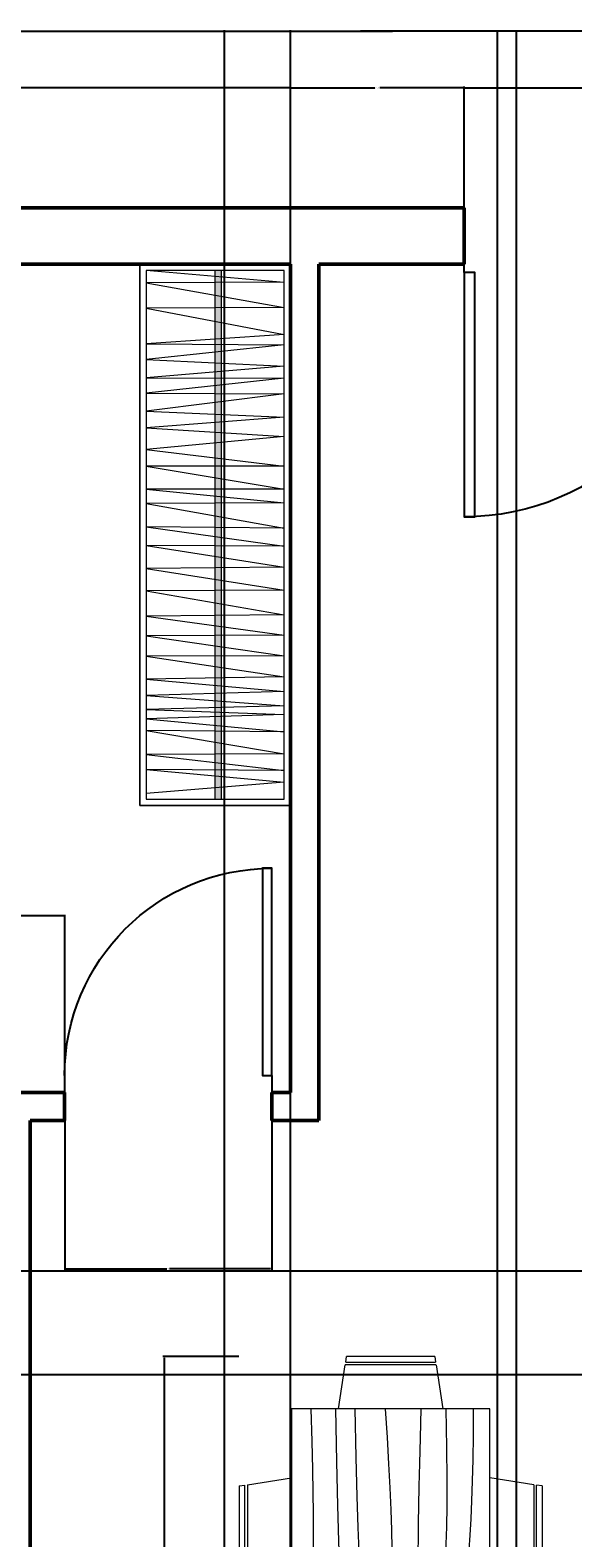
# Model space of a CAD drawing. Units: inches. Extents: x 1974 to 2406, y 1583 to 2170.
# Tile 5 of 6: x 2138 to 2224, y 1930 to 2170. Entities that reach past the tile are written whole.
import ezdxf

# ---------------------------------------------------------------- set-up
doc = ezdxf.new("R2010")
doc.units = ezdxf.units.IN
for name, color, linetype, lineweight in [('A-ANNO-DIMS', 2, 'Continuous', 18), ('A-FURN', 3, 'Continuous', 18), ('door', 60, 'Continuous', 25), ('wall', 240, 'Continuous', 50)]:
    doc.layers.add(name, color=color, linetype=linetype, lineweight=lineweight)
doc.layers.add('A-FLOR-CASE', color=40, linetype='Continuous', lineweight=18, true_color=0xf8d731)
doc.layers.add('A-FLOR-CASE-PATT', color=40, linetype='Continuous', lineweight=13, true_color=0xf8d731)
doc.styles.get("Standard").update_dxf_attribs({"font": 'arial.ttf'})
doc.dimstyles.get("Standard").update_dxf_attribs({"dimtxt": 0.18, "dimasz": 0.18, "dimexe": 0.18, "dimexo": 0.0625, "dimgap": 0.09, "dimtad": 0, "dimtih": 1, "dimtoh": 1, "dimdec": 4, "dimzin": 0, "dimdsep": 46, "dimtxsty": 'Standard', "dimcen": 0.09, "dimadec": 0, "dimazin": 0, "dimtfac": 1, "dimtdec": 4, "dimtofl": 0, "dimtmove": 0, "dimatfit": 3, "dimfxl": 1, "dimtolj": 1, "dimtzin": 0, "dimarcsym": 0})

# ---------------------------------------------------------------- blocks, each defined once
blk = doc.blocks.new('*U2')
for p, q in [((0, 0), (0, -6)), ((40, 0), (40, -6))]:
    blk.add_line(p, q)
blk.add_lwpolyline([(0, 0), (0, 40), (1.75, 40), (1.75, 0)], close=True)
blk.add_arc((0, 0), 40, 0, 90)
blk = doc.blocks.new('Dining Set - 36 x 72 in.')
for p, q in [((-22, 27.5), (-22.1562, 26.50042)), ((-22, 27.5), (-6, 27.5)), ((-5.8437, 26.49966), (-6, 27.5)), ((6, 27.5), (5.8438, 26.50042)), ((6, 27.5), (22, 27.5)), ((22.1563, 26.49966), (22, 27.5)), ((-22.2343, 26.00059), (-23.4847, 17.99762)), ((-22.2304, 26), (-5.7608, 26)), ((-5.8416, 26.5), (-22.1534, 26.5)), ((-4.5152, 17.99762), (-5.7655, 25.99926)), ((5.7657, 26.00059), (4.5153, 17.99762)), ((5.7696, 26), (22.2392, 26)), ((22.1584, 26.5), (5.8466, 26.5)), ((23.4848, 17.99762), (22.2345, 25.99926)), ((36, 18), (-36, 18)), ((-36, 18), (-36, -18)), ((36, -18), (36, 18)), ((-44.0006, 8.23428), (-35.9976, 9.48474)), ((-44, 8.23041), (-44, -8.23915)), ((44.0006, 8.23428), (35.9976, 9.48474)), ((44, 8.23041), (44, -8.23915)), ((-45.5, 8), (-44.5004, 8.15617)), ((-45.5, 8), (-45.5, -8)), ((-44.5, -8.15843), (-44.5, 8.15338)), ((44.5, -8.15843), (44.5, 8.15338)), ((45.5, 8), (44.5005, 8.15617)), ((45.5, 8), (45.5, -8)), ((-44.4997, -8.15631), (-45.5, -8)), ((44.4997, -8.15631), (45.5, -8)), ((-35.9976, -9.48476), (-43.9993, -8.2345)), ((35.9976, -9.48476), (43.9993, -8.2345)), ((-36, -18), (36, -18)), ((-22.2343, -26.0006), (-23.4847, -17.99762)), ((-4.5152, -17.99762), (-5.7655, -25.99928)), ((5.7657, -26.0006), (4.5153, -17.99762)), ((23.4848, -17.99762), (22.2345, -25.99928)), ((-22.2304, -26), (-5.7608, -26)), ((-22, -27.5), (-22.1562, -26.50044)), ((-5.8416, -26.5), (-22.1534, -26.5)), ((-5.8437, -26.49967), (-6, -27.5)), ((5.7696, -26), (22.2392, -26)), ((6, -27.5), (5.8438, -26.50044)), ((22.1584, -26.5), (5.8466, -26.5)), ((22.1563, -26.49967), (22, -27.5)), ((-22, -27.5), (-6, -27.5)), ((6, -27.5), (22, -27.5))]:
    blk.add_line(p, q)
for points in [[(-36, 15), (-31.1772, 14.97754), (-26.8079, 14.91406), (-22.8538, 14.81543), (-19.276, 14.6875), (-16.0362, 14.53613), (-13.0957, 14.36718), (-10.4159, 14.18652), (-7.9583, 14), (-5.6904, 13.81315), (-3.6035, 13.63021), (-1.6954, 13.45508), (0.0365, 13.29166), (1.5945, 13.14388), (2.9811, 13.01562), (4.1988, 12.9108), (5.25, 12.83333), (6.1393, 12.78613), (6.8802, 12.76823), (7.4883, 12.77767), (7.9792, 12.8125), (8.3685, 12.87077), (8.6719, 12.95052), (8.9049, 13.0498), (9.0833, 13.16666), (9.2205, 13.29899), (9.3216, 13.44401), (9.3895, 13.59879), (9.4271, 13.76041), (9.4373, 13.92594), (9.4232, 14.09245), (9.3875, 14.257), (9.3333, 14.41666), (9.2638, 14.56917), (9.1836, 14.71484), (9.0975, 14.85465), (9.0104, 14.98958), (8.9272, 15.1206), (8.8529, 15.2487), (8.7922, 15.37483), (8.75, 15.5), (8.7305, 15.62467), (8.7344, 15.74739), (8.7617, 15.86621), (8.8125, 15.97916), (8.8867, 16.08431), (8.9844, 16.17968), (9.1055, 16.26334), (9.25, 16.33333), (9.4189, 16.38802), (9.6172, 16.42708), (9.8506, 16.45052), (10.125, 16.45833), (10.4463, 16.45052), (10.8203, 16.42708), (11.2529, 16.38802), (11.75, 16.33333), (12.3184, 16.26318), (12.9694, 16.17838), (13.7151, 16.07991), (14.5677, 15.96875), (15.5395, 15.84586), (16.6426, 15.71224), (17.8893, 15.56884), (19.2917, 15.41666), (20.859, 15.25667), (22.5879, 15.08984), (24.4721, 14.91715), (26.5052, 14.73958), (28.6809, 14.5581), (30.9929, 14.3737), (33.4347, 14.18733), (36, 14)], [(-36, 10), (-28.9766, 10.14274), (-23.1725, 10.20442), (-18.4241, 10.19775), (-14.5677, 10.13541), (-11.4399, 10.03011), (-8.877, 9.89453), (-6.7154, 9.74137), (-4.7917, 9.58333), (-2.9698, 9.43082), (-1.2246, 9.28515), (0.4415, 9.14534), (2.026, 9.01041), (3.5266, 8.87939), (4.9408, 8.7513), (6.266, 8.62516), (7.5, 8.5), (8.6411, 8.37549), (9.6914, 8.2539), (10.6538, 8.13818), (11.5312, 8.03125), (12.3267, 7.93603), (13.043, 7.85547), (13.6831, 7.79248), (14.25, 7.75), (14.7471, 7.7303), (15.1797, 7.73307), (15.5537, 7.75732), (15.875, 7.80208), (16.1494, 7.86637), (16.3828, 7.94922), (16.5811, 8.04964), (16.75, 8.16666), (16.8944, 8.29915), (17.0143, 8.44531), (17.1089, 8.60319), (17.1771, 8.77083), (17.218, 8.94629), (17.2305, 9.1276), (17.2137, 9.31282), (17.1667, 9.5), (17.0895, 9.6875), (16.987, 9.875), (16.8649, 10.0625), (16.7292, 10.25), (16.5856, 10.4375), (16.4401, 10.625), (16.2985, 10.8125), (16.1667, 11), (16.05, 11.18733), (15.9518, 11.3737), (15.8752, 11.5581), (15.8229, 11.73958), (15.798, 11.91715), (15.8034, 12.08984), (15.842, 12.25667), (15.9167, 12.41666), (16.0295, 12.56836), (16.1784, 12.70833), (16.3605, 12.83268), (16.5729, 12.9375), (16.8127, 13.01888), (17.0768, 13.07291), (17.3625, 13.0957), (17.6667, 13.08333), (17.9894, 13.03312), (18.3418, 12.94726), (18.7382, 12.82918), (19.1927, 12.68229), (19.7195, 12.51001), (20.3327, 12.31575), (21.0465, 12.10294), (21.875, 11.875), (22.8357, 11.63354), (23.959, 11.37304), (25.2786, 11.08618), (26.8282, 10.76562), (28.6414, 10.40405), (30.752, 9.99414), (33.1936, 9.52856), (36, 9)], [(-36, 5.5), (-30.7157, 5.3348), (-26.069, 5.20963), (-21.9946, 5.11767), (-18.4271, 5.05208), (-15.3009, 5.00602), (-12.5508, 4.97265), (-10.1112, 4.94515), (-7.9167, 4.91666), (-5.909, 4.88167), (-4.0586, 4.83984), (-2.3429, 4.79215), (-0.7396, 4.73958), (0.7739, 4.6831), (2.22, 4.6237), (3.6213, 4.56233), (5, 4.5), (6.373, 4.43782), (7.7344, 4.3776), (9.0723, 4.32129), (10.375, 4.27083), (11.6309, 4.22819), (12.8281, 4.19531), (13.9551, 4.17415), (15, 4.16666), (15.954, 4.17448), (16.819, 4.19791), (17.6001, 4.23698), (18.3021, 4.29166), (18.9299, 4.36198), (19.4883, 4.44791), (19.9823, 4.54948), (20.4167, 4.66666), (20.7969, 4.79899), (21.1302, 4.94401), (21.4245, 5.09879), (21.6875, 5.26041), (21.9271, 5.42594), (22.1511, 5.59245), (22.3672, 5.757), (22.5834, 5.91666), (22.8065, 6.06868), (23.0404, 6.21093), (23.2879, 6.34147), (23.5521, 6.45833), (23.8358, 6.55957), (24.142, 6.64323), (24.4735, 6.70735), (24.8334, 6.75), (25.2235, 6.76969), (25.642, 6.76692), (26.0858, 6.74267), (26.5521, 6.69791), (27.0379, 6.63362), (27.5404, 6.55078), (28.0565, 6.45036), (28.5834, 6.33333), (29.1242, 6.19987), (29.7071, 6.04687), (30.3661, 5.87044), (31.1354, 5.66666), (32.0493, 5.43164), (33.142, 5.16146), (34.4475, 4.85221), (36, 4.5)], [(-36, -1), (-30.7915, -0.6591), (-26.0195, -0.38216), (-21.6519, -0.16284), (-17.6563, 0.00521), (-14.0005, 0.12833), (-10.6523, 0.21289), (-7.5796, 0.26522), (-4.75, 0.29166), (-2.134, 0.29793), (0.2878, 0.28711), (2.5317, 0.26163), (4.6146, 0.22396), (6.5529, 0.17651), (8.3633, 0.12174), (10.0623, 0.06209), (11.6667, 0), (13.1899, -0.06201), (14.6341, -0.1211), (15.9982, -0.17432), (17.2813, -0.21875), (18.4823, -0.25147), (19.6003, -0.26953), (20.6343, -0.27002), (21.5834, -0.25), (22.4481, -0.20768), (23.2357, -0.14584), (23.9549, -0.06836), (24.6146, 0.02083), (25.2235, 0.11784), (25.7904, 0.21875), (26.3241, 0.31966), (26.8334, 0.41666), (27.3265, 0.50618), (27.8099, 0.58593), (28.2894, 0.65397), (28.7709, 0.70833), (29.2601, 0.74707), (29.763, 0.76823), (30.2855, 0.76985), (30.8334, 0.75), (31.4088, 0.70784), (31.9994, 0.64713), (32.589, 0.57275), (33.1615, 0.48958), (33.7008, 0.4025), (34.1908, 0.3164), (34.6153, 0.23616), (34.9584, 0.16666), (35.2099, 0.11165), (35.3848, 0.07031), (35.504, 0.04069), (35.5886, 0.02083), (35.6594, 0.00879), (35.7377, 0.0026), (35.8442, 0.00032), (36, 0)], [(-36, -6.5), (-27.1843, -6.31267), (-20.084, -6.1263), (-14.469, -5.9419), (-10.1094, -5.76042), (-6.7752, -5.58285), (-4.2363, -5.41016), (-2.2629, -5.24333), (-0.625, -5.08334), (0.8708, -4.93099), (2.2715, -4.78646), (3.5872, -4.64974), (4.8281, -4.52084), (6.0046, -4.39974), (7.127, -4.28646), (8.2053, -4.18099), (9.25, -4.08334), (10.2705, -3.99382), (11.2734, -3.91407), (12.2647, -3.84603), (13.25, -3.79167), (14.2354, -3.75293), (15.2266, -3.73177), (16.2295, -3.73015), (17.25, -3.75), (18.2912, -3.79248), (19.3451, -3.85547), (20.4009, -3.93604), (21.4479, -4.03125), (22.4754, -4.13819), (23.4727, -4.25391), (24.4289, -4.37549), (25.3334, -4.5), (26.1785, -4.62492), (26.9694, -4.74935), (27.7145, -4.87281), (28.4219, -4.99479), (29.1, -5.11483), (29.7572, -5.23242), (30.4016, -5.34709), (31.0417, -5.45834), (31.6837, -5.56437), (32.3262, -5.65821), (32.9658, -5.73153), (33.599, -5.77604), (34.2224, -5.78345), (34.8327, -5.74545), (35.4264, -5.65373), (36, -5.5)], [(-36, -10), (-26.4022, -9.81299), (-18.4675, -9.62891), (-11.9839, -9.45069), (-6.7396, -9.28125), (-2.5226, -9.12354), (0.8789, -8.98047), (3.6769, -8.85498), (6.0833, -8.75), (8.2767, -8.66765), (10.3021, -8.60677), (12.1712, -8.56543), (13.8958, -8.54167), (15.4876, -8.53353), (16.9583, -8.53907), (18.3197, -8.55632), (19.5834, -8.58334), (20.7616, -8.61841), (21.8685, -8.66081), (22.9188, -8.71004), (23.9271, -8.76563), (24.9081, -8.82707), (25.8763, -8.89388), (26.8465, -8.96558), (27.8334, -9.04167), (28.8474, -9.12118), (29.8828, -9.20117), (30.93, -9.27824), (31.9792, -9.34896), (33.0205, -9.40991), (34.0443, -9.45768), (35.0407, -9.48885), (36, -9.5)], [(-36, -14.5), (-30.0881, -14.33513), (-25.0332, -14.21224), (-20.7312, -14.12647), (-17.0781, -14.07292), (-13.97, -14.04671), (-11.3027, -14.04297), (-8.9724, -14.05681), (-6.875, -14.08334), (-4.9224, -14.11833), (-3.0905, -14.16016), (-1.3709, -14.20785), (0.2448, -14.26042), (1.7647, -14.3169), (3.1973, -14.3763), (4.5507, -14.43767), (5.8333, -14.5), (7.0554, -14.5621), (8.235, -14.62175), (9.3922, -14.67652), (10.5469, -14.72396), (11.7192, -14.76164), (12.929, -14.78711), (14.1965, -14.79794), (15.5417, -14.79167), (16.9933, -14.76424), (18.6152, -14.70508), (20.4804, -14.60197), (22.6615, -14.44271), (25.2312, -14.21509), (28.2624, -13.9069), (31.8277, -13.50594), (36, -13)]]:
    blk.add_lwpolyline(points)
blk = doc.blocks.new('CLOSET-HANGER-RUN')
for p, q in [((0, 0), (0, 22)), ((0.94, 0), (2.86, 22)), ((2.86, 22), (2.99, 0)), ((2.99, 0), (6.93, 22)), ((6.93, 22), (6.99, 0)), ((6.99, 0), (11.19, 22)), ((11.19, 22), (12.71, 0)), ((12.71, 0), (12.83, 22)), ((12.83, 22), (15.2, 0)), ((15.2, 0), (16.24, 22)), ((16.24, 22), (18.1, 0)), ((18.1, 0), (18.16, 22)), ((18.16, 22), (20.55, 0)), ((20.55, 0), (20.68, 22)), ((20.68, 22), (23.44, 0)), ((23.44, 0), (24.36, 22)), ((24.36, 22), (26.08, 0)), ((26.08, 0), (27.44, 22)), ((27.44, 22), (29.52, 0)), ((29.52, 0), (32.2, 22)), ((32.2, 22), (32.2, 0)), ((32.2, 0), (35.87, 22)), ((35.87, 22), (35.87, 0)), ((35.87, 0), (38.02, 22)), ((38.02, 22), (38.12, 0)), ((38.12, 0), (42.07, 22)), ((42.07, 22), (41.87, 0)), ((41.87, 0), (44.93, 22)), ((44.93, 22), (44.83, 0)), ((44.83, 0), (48.29, 22)), ((48.29, 22), (48.48, 0)), ((48.48, 0), (51.94, 22)), ((51.94, 22), (52.04, 0)), ((52.04, 0), (55.89, 22)), ((55.89, 22), (56.08, 0)), ((56.08, 0), (59.14, 22)), ((59.14, 22), (59.24, 0)), ((59.24, 0), (62.4, 22)), ((62.4, 22), (62.5, 0)), ((62.5, 0), (65.76, 22)), ((65.76, 22), (66.15, 0)), ((66.15, 0), (68.13, 22)), ((68.13, 22), (68.72, 0)), ((68.72, 0), (70.4, 22)), ((70.4, 22), (70.99, 0)), ((70.99, 0), (71.78, 22)), ((71.78, 22), (72.44, 0))]:
    blk.add_line(p, q)
blk = doc.blocks.new('*D42')
at = {"layer": 'A-ANNO-DIMS', "color": 0, "lineweight": -2, "transparency": 16777216}
for p, q in [((2170.92, 1958.88), (2158.82, 1958.88)), ((2159, 1958.7), (2159, 1919.13)), ((2159, 1879.18), (2159, 1918.76)), ((2170.92, 1879), (2158.82, 1879))]:
    blk.add_line(p, q, dxfattribs=at)
at = {"layer": 'A-ANNO-DIMS', "color": 0, "transparency": 16777216}
for points in [[(2158.97, 1958.7), (2159.03, 1958.7), (2159, 1958.88)], [(2158.97, 1879.18), (2159.03, 1879.18), (2159, 1879)]]:
    blk.add_solid(points, dxfattribs=at)
at = {"layer": 'Defpoints', "color": 0, "transparency": 16777216}
for p in [(2170.98, 1958.88), (2159, 1879), (2170.98, 1879)]:
    blk.add_point(p, dxfattribs=at)
at = {"layer": 'A-ANNO-DIMS', "color": 0, "transparency": 16777216, "insert": (2159, 1918.94), "char_height": 0.18, "attachment_point": 5}
blk.add_mtext('\\A1;DINING SET 80', dxfattribs=at)
blk = doc.blocks.new('*D48')
at = {"layer": 'A-ANNO-DIMS', "color": 0, "lineweight": -2, "transparency": 16777216}
for p, q in [((2002.16, 2142.05), (2002.16, 2170.29)), ((2002.34, 2170.11), (2189.51, 2170.11)), ((2377.48, 2170.11), (2190.3, 2170.11)), ((2377.66, 2142.05), (2377.66, 2170.29))]:
    blk.add_line(p, q, dxfattribs=at)
at = {"layer": 'A-ANNO-DIMS', "color": 0, "transparency": 16777216}
for points in [[(2002.34, 2170.14), (2002.34, 2170.08), (2002.16, 2170.11)], [(2377.48, 2170.14), (2377.48, 2170.08), (2377.66, 2170.11)]]:
    blk.add_solid(points, dxfattribs=at)
at = {"layer": 'Defpoints', "color": 0, "transparency": 16777216}
for p in [(2377.66, 2170.11), (2002.16, 2141.99), (2377.66, 2141.99)]:
    blk.add_point(p, dxfattribs=at)
at = {"layer": 'A-ANNO-DIMS', "color": 0, "transparency": 16777216, "insert": (2189.91, 2170.11), "char_height": 0.18, "attachment_point": 5}
blk.add_mtext('\\A1;375.5', dxfattribs=at)
blk = doc.blocks.new('*D50')
at = {"layer": 'A-ANNO-DIMS', "color": 0, "lineweight": -2, "transparency": 16777216}
for p, q in [((2011.16, 2133.05), (2011.16, 2161.29)), ((2011.34, 2161.11), (2094.88, 2161.11)), ((2178.98, 2161.11), (2095.44, 2161.11)), ((2179.16, 2133.05), (2179.16, 2161.29))]:
    blk.add_line(p, q, dxfattribs=at)
at = {"layer": 'A-ANNO-DIMS', "color": 0, "transparency": 16777216}
for points in [[(2011.34, 2161.14), (2011.34, 2161.08), (2011.16, 2161.11)], [(2178.98, 2161.14), (2178.98, 2161.08), (2179.16, 2161.11)]]:
    blk.add_solid(points, dxfattribs=at)
at = {"layer": 'Defpoints', "color": 0, "transparency": 16777216}
for p in [(2179.16, 2161.11), (2011.16, 2132.99), (2179.16, 2132.99)]:
    blk.add_point(p, dxfattribs=at)
at = {"layer": 'A-ANNO-DIMS', "color": 0, "transparency": 16777216, "insert": (2095.16, 2161.11), "char_height": 0.18, "attachment_point": 5}
blk.add_mtext('\\A1;168', dxfattribs=at)
blk = doc.blocks.new('*D51')
at = {"layer": 'A-ANNO-DIMS', "color": 0, "lineweight": -2, "transparency": 16777216}
for p, q in [((2179.16, 2133.05), (2179.16, 2161.29)), ((2179.34, 2161.11), (2192.59, 2161.11)), ((2206.64, 2161.11), (2193.38, 2161.11)), ((2206.82, 2133.05), (2206.82, 2161.29))]:
    blk.add_line(p, q, dxfattribs=at)
at = {"layer": 'A-ANNO-DIMS', "color": 0, "transparency": 16777216}
for points in [[(2179.34, 2161.14), (2179.34, 2161.08), (2179.16, 2161.11)], [(2206.64, 2161.14), (2206.64, 2161.08), (2206.82, 2161.11)]]:
    blk.add_solid(points, dxfattribs=at)
at = {"layer": 'Defpoints', "color": 0, "transparency": 16777216}
for p in [(2206.82, 2161.11), (2179.16, 2132.99), (2206.82, 2132.99)]:
    blk.add_point(p, dxfattribs=at)
at = {"layer": 'A-ANNO-DIMS', "color": 0, "transparency": 16777216, "insert": (2192.99, 2161.11), "char_height": 0.18, "attachment_point": 5}
blk.add_mtext('\\A1;27.66', dxfattribs=at)
blk = doc.blocks.new('*D52')
at = {"layer": 'A-ANNO-DIMS', "color": 0, "lineweight": -2, "transparency": 16777216}
for p, q in [((2206.82, 2133.05), (2206.82, 2161.29)), ((2207, 2161.11), (2226.1, 2161.11)), ((2245.64, 2161.11), (2226.54, 2161.11)), ((2245.82, 2133.05), (2245.82, 2161.29))]:
    blk.add_line(p, q, dxfattribs=at)
at = {"layer": 'A-ANNO-DIMS', "color": 0, "transparency": 16777216}
for points in [[(2207, 2161.14), (2207, 2161.08), (2206.82, 2161.11)], [(2245.64, 2161.14), (2245.64, 2161.08), (2245.82, 2161.11)]]:
    blk.add_solid(points, dxfattribs=at)
at = {"layer": 'Defpoints', "color": 0, "transparency": 16777216}
for p in [(2245.82, 2161.11), (2206.82, 2132.99), (2245.82, 2132.99)]:
    blk.add_point(p, dxfattribs=at)
at = {"layer": 'A-ANNO-DIMS', "color": 0, "transparency": 16777216, "insert": (2226.32, 2161.11), "char_height": 0.18, "attachment_point": 5}
blk.add_mtext('\\A1;39', dxfattribs=at)
blk = doc.blocks.new('*D68')
at = {"layer": 'A-ANNO-DIMS', "color": 0, "lineweight": -2, "transparency": 16777216}
for p, q in [((2143.16, 2000.93), (2143.16, 1972.69)), ((2176.16, 2000.93), (2176.16, 1972.69)), ((2143.34, 1972.87), (2159.44, 1972.87)), ((2175.98, 1972.87), (2159.88, 1972.87))]:
    blk.add_line(p, q, dxfattribs=at)
at = {"layer": 'A-ANNO-DIMS', "color": 0, "transparency": 16777216}
for points in [[(2143.34, 1972.9), (2143.34, 1972.84), (2143.16, 1972.87)], [(2175.98, 1972.9), (2175.98, 1972.84), (2176.16, 1972.87)]]:
    blk.add_solid(points, dxfattribs=at)
at = {"layer": 'Defpoints', "color": 0, "transparency": 16777216}
for p in [(2143.16, 2000.99), (2176.16, 2000.99), (2143.16, 1972.87)]:
    blk.add_point(p, dxfattribs=at)
at = {"layer": 'A-ANNO-DIMS', "color": 0, "transparency": 16777216, "insert": (2159.66, 1972.87), "char_height": 0.18, "attachment_point": 5}
blk.add_mtext('\\A1;33', dxfattribs=at)
blk = doc.blocks.new('*D69')
at = {"layer": 'A-ANNO-DIMS', "color": 0, "lineweight": -2, "transparency": 16777216}
for p, q in [((2091.94, 2001.05), (2091.94, 2029.29)), ((2092.12, 2029.11), (2117.16, 2029.11)), ((2142.98, 2029.11), (2117.94, 2029.11)), ((2143.16, 2001.05), (2143.16, 2029.29))]:
    blk.add_line(p, q, dxfattribs=at)
at = {"layer": 'A-ANNO-DIMS', "color": 0, "transparency": 16777216}
for points in [[(2092.12, 2029.14), (2092.12, 2029.08), (2091.94, 2029.11)], [(2142.98, 2029.14), (2142.98, 2029.08), (2143.16, 2029.11)]]:
    blk.add_solid(points, dxfattribs=at)
at = {"layer": 'Defpoints', "color": 0, "transparency": 16777216}
for p in [(2143.16, 2029.11), (2091.94, 2000.99), (2143.16, 2000.99)]:
    blk.add_point(p, dxfattribs=at)
at = {"layer": 'A-ANNO-DIMS', "color": 0, "transparency": 16777216, "insert": (2117.55, 2029.11), "char_height": 0.18, "attachment_point": 5}
blk.add_mtext('\\A1;51.22', dxfattribs=at)
blk = doc.blocks.new('*D73')
at = {"layer": 'A-ANNO-DIMS', "color": 0, "lineweight": -2, "transparency": 16777216}
for p, q in [((2258.6, 1972.49), (1973.86, 1972.49)), ((1974.04, 1972.31), (1974.04, 1941.67)), ((1974.04, 1910.67), (1974.04, 1941.31)), ((2254.1, 1910.49), (1973.86, 1910.49))]:
    blk.add_line(p, q, dxfattribs=at)
at = {"layer": 'A-ANNO-DIMS', "color": 0, "transparency": 16777216}
for points in [[(1974.01, 1972.31), (1974.07, 1972.31), (1974.04, 1972.49)], [(1974.01, 1910.67), (1974.07, 1910.67), (1974.04, 1910.49)]]:
    blk.add_solid(points, dxfattribs=at)
at = {"layer": 'Defpoints', "color": 0, "transparency": 16777216}
for p in [(2258.66, 1972.49), (1974.04, 1910.49), (2254.16, 1910.49)]:
    blk.add_point(p, dxfattribs=at)
at = {"layer": 'A-ANNO-DIMS', "color": 0, "transparency": 16777216, "insert": (1974.04, 1941.49), "char_height": 0.18, "attachment_point": 5}
blk.add_mtext('\\A1;62', dxfattribs=at)
blk = doc.blocks.new('*D81')
at = {"layer": 'A-ANNO-DIMS', "color": 0, "lineweight": -2, "transparency": 16777216}
for p, q in [((2258.6, 1972.49), (1973.86, 1972.49)), ((1974.04, 1972.31), (1974.04, 1964.42)), ((1974.04, 1956.17), (1974.04, 1964.06)), ((2258.6, 1955.99), (1973.86, 1955.99))]:
    blk.add_line(p, q, dxfattribs=at)
at = {"layer": 'A-ANNO-DIMS', "color": 0, "transparency": 16777216}
for points in [[(1974.01, 1972.31), (1974.07, 1972.31), (1974.04, 1972.49)], [(1974.01, 1956.17), (1974.07, 1956.17), (1974.04, 1955.99)]]:
    blk.add_solid(points, dxfattribs=at)
at = {"layer": 'Defpoints', "color": 0, "transparency": 16777216}
for p in [(1974.04, 1972.49), (2258.66, 1972.49), (2258.66, 1955.99)]:
    blk.add_point(p, dxfattribs=at)
at = {"layer": 'A-ANNO-DIMS', "color": 0, "transparency": 16777216, "insert": (1974.04, 1964.24), "char_height": 0.18, "attachment_point": 5}
blk.add_mtext('\\A1;16.5', dxfattribs=at)
blk = doc.blocks.new('*D89')
at = {"layer": 'A-ANNO-DIMS', "color": 0, "lineweight": -2, "transparency": 16777216}
for p, q in [((2179.16, 1809.05), (2179.16, 2170.29)), ((2179.34, 2170.11), (2195.44, 2170.11)), ((2211.98, 2170.11), (2195.88, 2170.11)), ((2212.16, 1809.05), (2212.16, 2170.29))]:
    blk.add_line(p, q, dxfattribs=at)
at = {"layer": 'A-ANNO-DIMS', "color": 0, "transparency": 16777216}
for points in [[(2179.34, 2170.14), (2179.34, 2170.08), (2179.16, 2170.11)], [(2211.98, 2170.14), (2211.98, 2170.08), (2212.16, 2170.11)]]:
    blk.add_solid(points, dxfattribs=at)
at = {"layer": 'Defpoints', "color": 0, "transparency": 16777216}
for p in [(2212.16, 2170.11), (2179.16, 1808.99), (2212.16, 1808.99)]:
    blk.add_point(p, dxfattribs=at)
at = {"layer": 'A-ANNO-DIMS', "color": 0, "transparency": 16777216, "insert": (2195.66, 2170.11), "char_height": 0.18, "attachment_point": 5}
blk.add_mtext('\\A1;33', dxfattribs=at)
blk = doc.blocks.new('*D92')
at = {"layer": 'A-ANNO-DIMS', "color": 0, "lineweight": -2, "transparency": 16777216}
for p, q in [((2168.64, 1725.52), (2168.64, 2170.29)), ((2168.82, 2170.11), (2191.5, 2170.11)), ((2214.98, 2170.11), (2192.3, 2170.11)), ((2215.16, 1728.05), (2215.16, 2170.29))]:
    blk.add_line(p, q, dxfattribs=at)
at = {"layer": 'A-ANNO-DIMS', "color": 0, "transparency": 16777216}
for points in [[(2168.82, 2170.14), (2168.82, 2170.08), (2168.64, 2170.11)], [(2214.98, 2170.14), (2214.98, 2170.08), (2215.16, 2170.11)]]:
    blk.add_solid(points, dxfattribs=at)
at = {"layer": 'Defpoints', "color": 0, "transparency": 16777216}
for p in [(2215.16, 2170.11), (2215.16, 1727.99), (2168.64, 1725.46)]:
    blk.add_point(p, dxfattribs=at)
at = {"layer": 'A-ANNO-DIMS', "color": 0, "transparency": 16777216, "insert": (2191.9, 2170.11), "char_height": 0.18, "attachment_point": 5}
blk.add_mtext('\\A1;46.52', dxfattribs=at)

msp = doc.modelspace()

# ---------------------------------------------------------------- hatches: boundary and pattern name
at = {"layer": 'A-FLOR-CASE-PATT'}
h = msp.add_hatch(color=256, dxfattribs=at)
h.dxf.hatch_style = 1
h.paths.add_polyline_path([(2168.1581, 2131.9921), (2167.1581, 2131.9921), (2167.1581, 2047.7367), (2168.1581, 2047.7367)])

# ---------------------------------------------------------------- linework, layer by layer
at = {"layer": 'A-FLOR-CASE'}
for p, q in [((2155.1581, 2046.7367), (2155.1581, 2132.9921)), ((2167.1581, 2047.7367), (2167.1581, 2131.9921)), ((2168.1581, 2047.7367), (2168.1581, 2131.9921)), ((2156.1581, 2060.5488), (2178.1581, 2058.475)), ((2178.1581, 2058.475), (2156.1581, 2058.6733)), ((2156.1581, 2058.6733), (2178.1581, 2054.9552)), ((2178.1581, 2054.9552), (2156.1581, 2054.856)), ((2156.1581, 2054.856), (2178.1581, 2052.2782)), ((2178.1581, 2052.2782), (2156.1581, 2052.4269)), ((2156.1581, 2052.4269), (2178.1581, 2050.4439)), ((2178.1581, 2050.4439), (2156.1581, 2048.6097)), ((2179.1581, 2046.7367), (2155.1581, 2046.7367))]:
    msp.add_line(p, q, dxfattribs=at)
for points in [[(2179.1581, 2132.9921), (2155.1581, 2132.9921), (2155.1581, 2046.7367), (2179.1581, 2046.7367)], [(2178.1581, 2131.9921), (2156.1581, 2131.9921), (2156.1581, 2047.7367), (2178.1581, 2047.7367)]]:
    msp.add_lwpolyline(points, close=True, dxfattribs=at)
at = {"layer": 'wall'}
for p, q in [((2002.1581, 2141.9921), (2206.8193, 2141.9921)), ((2206.8193, 2132.9921), (2206.8193, 2141.9921)), ((2011.1581, 2132.9921), (2179.1581, 2132.9921)), ((2179.1581, 2132.9921), (2179.1581, 2000.9921)), ((2183.6581, 2132.9921), (2183.6581, 1996.4921)), ((2183.6581, 2132.9921), (2206.8193, 2132.9921)), ((2183.6581, 2132.9921), (2206.8193, 2132.9921)), ((2091.9418, 2000.9921), (2143.1581, 2000.9921)), ((2143.1581, 2000.9921), (2143.1581, 1996.4921)), ((2179.1581, 2000.9921), (2176.1581, 2000.9921)), ((2179.1581, 2000.9921), (2176.1581, 2000.9921)), ((2176.1581, 2000.9921), (2176.1581, 1996.4921)), ((2176.1581, 2000.9921), (2179.1581, 2000.9921)), ((2137.6581, 1996.4921), (2137.6581, 1844.9921)), ((2137.6581, 1996.4921), (2143.1581, 1996.4921)), ((2176.1581, 1996.4921), (2183.6581, 1996.4921))]:
    msp.add_line(p, q, dxfattribs=at)

# ---------------------------------------------------------------- block references
at = {"layer": 'A-FLOR-CASE', "rotation": 270.000000000005}
msp.add_blockref('CLOSET-HANGER-RUN', (2156.1579, 2132.9921), dxfattribs=at)
at = {"layer": 'A-FURN', "xscale": 0.8778001079660128, "yscale": 0.8778001079660128, "zscale": 0.8778001079660128, "rotation": 270}
msp.add_blockref('Dining Set - 36 x 72 in.', (2195.122, 1918.9446), dxfattribs=at)
at = {"layer": 'door', "xscale": -0.9732547723877202, "yscale": 0.9732547723877202, "zscale": 0.9732547723877202, "rotation": 180}
msp.add_blockref('*U2', (2206.8193, 2131.6526), dxfattribs=at)
at = {"layer": 'door', "xscale": -0.8252274917434117, "yscale": 0.8252274917434117, "zscale": 0.8252274917434117}
msp.add_blockref('*U2', (2176.1581, 2003.6935), dxfattribs=at)

# ---------------------------------------------------------------- dimensions: what is measured, and where the dimension line sits
at = {"layer": 'A-ANNO-DIMS'}
for base, p1, p2, override, picture, middle in [((2377.6581, 2170.1096), (2002.1581, 2141.9921), (2377.6581, 2141.9921), {"dimdec": 1, "dimlfac": 1, "dimrnd": 0, "dimzin": 0, "dimdsep": 46, "dimlunit": 2}, '*D48', (2189.9081, 2170.1096)), ((2215.1581, 2170.1096), (2168.6394, 1725.4624), (2215.1581, 1727.9921), {"dimdec": 2, "dimlfac": 1, "dimrnd": 0, "dimzin": 0, "dimdsep": 46, "dimlunit": 2}, '*D92', (2191.8987, 2170.1096)), ((2212.1581, 2170.1096), (2179.1581, 1808.9921), (2212.1581, 1808.9921), {"dimdec": 0, "dimlfac": 1, "dimrnd": 0, "dimzin": 0, "dimdsep": 46, "dimlunit": 2}, '*D89', (2195.6581, 2170.1096)), ((2179.1581, 2161.1096), (2011.1581, 2132.9921), (2179.1581, 2132.9921), {"dimdec": 0, "dimlfac": 1, "dimrnd": 0, "dimzin": 0, "dimdsep": 46, "dimlunit": 2}, '*D50', (2095.1581, 2161.1096)), ((2245.8193, 2161.1096), (2206.8193, 2132.9921), (2245.8193, 2132.9921), {"dimdec": 0, "dimlfac": 1, "dimrnd": 0, "dimzin": 0, "dimdsep": 46, "dimlunit": 2}, '*D52', (2226.3193, 2161.1096)), ((2143.1581, 2029.1096), (2091.9418, 2000.9921), (2143.1581, 2000.9921), {"dimdec": 2, "dimlfac": 1, "dimrnd": 0, "dimzin": 0, "dimdsep": 46, "dimlunit": 2}, '*D69', (2117.5499, 2029.1096))]:
    dim = msp.add_linear_dim(base=base, p1=p1, p2=p2, dimstyle='Standard', override=override, dxfattribs=at)
    dim.commit()
    dim.dimension.update_dxf_attribs({"geometry": picture, "text_midpoint": middle})
for base, p1, p2, angle, override, picture, middle in [((2206.8193, 2161.1096), (2179.1581, 2132.9921), (2206.8193, 2132.9921), 0, {"dimdec": 2, "dimlfac": 1, "dimrnd": 0, "dimzin": 0, "dimdsep": 46, "dimlunit": 2}, '*D51', (2192.9887, 2161.1096)), ((2143.1581, 1972.8746), (2176.1581, 2000.9921), (2143.1581, 2000.9921), 180, {"dimdec": 0, "dimlfac": 1, "dimrnd": 0, "dimzin": 0, "dimdsep": 46, "dimlunit": 2}, '*D68', (2159.6581, 1972.8746)), ((1974.0406, 1972.4921), (2258.6581, 1955.9921), (2258.6581, 1972.4921), 90, {"dimdec": 1, "dimlfac": 1, "dimrnd": 0, "dimzin": 0, "dimdsep": 46, "dimlunit": 2}, '*D81', (1974.0406, 1964.2421)), ((1974.0406, 1910.4921), (2258.6581, 1972.4921), (2254.1581, 1910.4921), 90, {"dimdec": 0, "dimlfac": 1, "dimrnd": 0, "dimzin": 0, "dimdsep": 46, "dimlunit": 2}, '*D73', (1974.0406, 1941.4921))]:
    dim = msp.add_linear_dim(base=base, p1=p1, p2=p2, angle=angle, dimstyle='Standard', override=override, dxfattribs=at)
    dim.commit()
    dim.dimension.update_dxf_attribs({"geometry": picture, "text_midpoint": middle})
dim = msp.add_linear_dim(base=(2159.0005, 1879.0047), p1=(2170.9825, 1958.8845), p2=(2170.9825, 1879.0047), angle=270, text='DINING SET <>', dimstyle='Standard', override={"dimdec": 0, "dimlfac": 1, "dimrnd": 0, "dimzin": 0, "dimdsep": 46, "dimlunit": 2}, dxfattribs=at)
dim.commit()
dim.dimension.update_dxf_attribs({"geometry": '*D42', "text_midpoint": (2159.0005, 1918.9446)})

doc.saveas('drawing.dxf')
